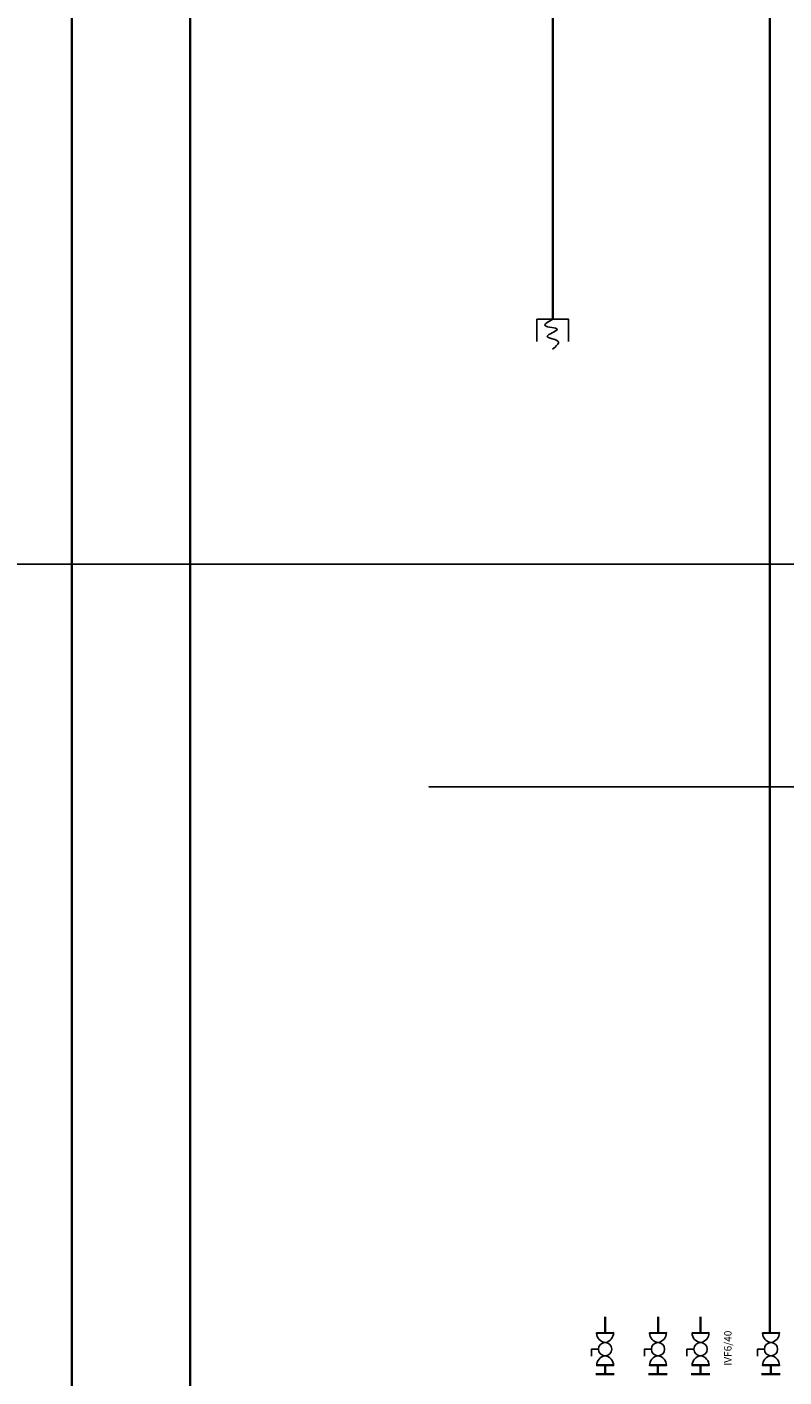
# Model space of a CAD drawing. Units: millimetres. Extents: x 353872 to 441597, y 126154 to 187356.
# Tile 11 of 28: x 381210 to 391248, y 149281 to 167178. Entities that reach past the tile are written whole.
import ezdxf

# ---------------------------------------------------------------- set-up
doc = ezdxf.new("R2010")
doc.units = ezdxf.units.MM
doc.linetypes.add('ACAD_ISO02W100', pattern=[15, 12, -3])
for name, color, linetype, lineweight in [('A-ANNO-DIMS', 2, 'Continuous', 18), ('P-ANNO-TEXT', 7, 'Continuous', 25), ('P-BNDY', 4, 'ACAD_ISO02W100', 25), ('P-PIPE', 3, 'Continuous', 35), ('P-VALV', 2, 'Continuous', 25)]:
    doc.layers.add(name, color=color, linetype=linetype, lineweight=lineweight)
doc.styles.get("Standard").update_dxf_attribs({"font": 'arial.ttf'})
doc.dimstyles.get("Standard").update_dxf_attribs({"dimtxt": 0.18, "dimasz": 0.18, "dimexe": 0.18, "dimexo": 0.0625, "dimgap": 0.09, "dimtad": 0, "dimtih": 1, "dimtoh": 1, "dimdec": 4, "dimzin": 0, "dimdsep": 46, "dimtxsty": 'Standard', "dimcen": 0.09, "dimadec": 0, "dimazin": 0, "dimtfac": 1, "dimtdec": 4, "dimtofl": 0, "dimtmove": 0, "dimatfit": 3, "dimfxl": 1, "dimtolj": 1, "dimtzin": 0, "dimarcsym": 0})

# ---------------------------------------------------------------- blocks, each defined once
blk = doc.blocks.new('VALVE-C')
for points in [[(0, 8), (224, 8)], [(0, 5), (224, 5)], [(0, 3), (0, 0), (224, 0), (224, 3)], [(0, 3), (0, 3), (222, 3), (224, 3)]]:
    blk.add_lwpolyline(points)
for centre, start, end in [((128, 1), 97.3612, 180.5798), ((96, 2), 359.2193, 82.8397)]:
    blk.add_arc(centre, 128, start, end)
blk = doc.blocks.new('*D34')
at = {"layer": 'A-ANNO-DIMS', "color": 0, "lineweight": -2, "transparency": 16777216}
for p, q in [((399457, 167930), (356736, 167930)), ((356737, 167930), (356737, 163994)), ((356737, 160058), (356737, 163994)), ((399457, 160058), (356736, 160058))]:
    blk.add_line(p, q, dxfattribs=at)
at = {"layer": 'A-ANNO-DIMS', "color": 0, "transparency": 16777216}
for points in [[(356737, 167930), (356737, 167930), (356737, 167930)], [(356737, 160058), (356737, 160058), (356737, 160058)]]:
    blk.add_solid(points, dxfattribs=at)
at = {"layer": 'Defpoints', "color": 0, "transparency": 16777216}
for p in [(399457, 167930), (356737, 160058), (399457, 160058)]:
    blk.add_point(p, dxfattribs=at)
at = {"layer": 'A-ANNO-DIMS', "color": 0, "transparency": 16777216, "insert": (356737, 163994), "char_height": 0.18, "attachment_point": 5}
blk.add_mtext('\\A1;7872', dxfattribs=at)

msp = doc.modelspace()

# ---------------------------------------------------------------- linework, layer by layer
at = {"layer": 'P-BNDY'}
msp.add_line((436591, 157104.68), (386532.91, 157104.68), dxfattribs=at)
at = {"layer": 'P-PIPE'}
for p, q in [((388876.24, 150079.91), (388876.24, 149867.25)), ((389577.76, 150079.91), (389577.76, 149867.25)), ((390142.2, 150079.91), (390142.2, 149867.25)), ((391060.3, 150079.91), (391060.3, 149867.25)), ((388996.7, 149319.73), (388751.94, 149319.73)), ((388874.98, 149433.14), (388874.98, 149319.73)), ((389698.22, 149319.73), (389453.46, 149319.73)), ((389576.5, 149433.14), (389576.5, 149319.73)), ((390262.67, 149319.73), (390017.91, 149319.73)), ((390140.95, 149433.14), (390140.95, 149319.73)), ((391196.72, 149319.73), (390951.96, 149319.73)), ((391075, 149433.14), (391075, 149319.73))]:
    msp.add_line(p, q, dxfattribs=at)
for points in [[(391060.3, 150079.91), (391060.3, 182028.44), (390103.2, 182028.44), (366976.76, 182028.44)], [(366976.76, 173434.34), (386613.67, 173434.34), (388181.19, 173434.34), (388181.19, 163303.71)], [(366976.76, 171744.89), (381803.29, 171744.89), (381803.29, 150820.94), (381803.29, 147742.48), (377889.79, 147742.48)]]:
    msp.add_lwpolyline(points, dxfattribs=at)
msp.add_lwpolyline([(388213.21, 147045.52), (383375.2, 147045.17), (383375.2, 147045.17), (383375.2, 149602.24), (383375.2, 167832.6), (382147.59, 167832.6, 1), (381458.98, 167832.6), (380124.81, 167832.6, 1), (379436.2, 167832.6), (368453.37, 167832.6)], format="xyb", dxfattribs=at)
at = {"layer": 'P-VALV'}
for points in [[(388391.21, 163010.43), (388391.21, 163303.71), (387971.17, 163303.71), (387971.17, 163010.43)], [(388787.65, 149650.19), (388695.2, 149650.19), (388695.2, 149559.43)], [(389489.17, 149650.19), (389396.73, 149650.19), (389396.73, 149559.43)], [(390053.62, 149650.19), (389961.17, 149650.19), (389961.17, 149559.43)], [(390987.67, 149650.19), (390895.22, 149650.19), (390895.22, 149559.43)]]:
    msp.add_lwpolyline(points, dxfattribs=at)
for centre in [(388875.94, 149650.19), (389577.46, 149650.19), (390141.91, 149650.19), (391075.95, 149650.19)]:
    msp.add_circle(centre, 88.29, dxfattribs=at)
msp.add_open_spline([(388181.19, 163303.71), (388122.73, 163271.25), (387989.49, 163197.29), (388375.07, 163190.34), (387981.2, 163061.46), (388331.17, 163032.41), (388225.96, 162945.08), (388179.78, 162906.75)], degree=3, knots=[0, 0, 0, 0, 131.62046813, 299.94883433, 460.08690619, 621.6605897, 748.04024912, 748.04024912, 748.04024912, 748.04024912], dxfattribs=at)

# ---------------------------------------------------------------- block references
for p, rotation in [((388987.77, 149869.79), 181.3019170023728), ((389689.29, 149869.79), 181.3019170023652), ((390253.73, 149869.79), 181.3019170023652), ((391187.78, 149869.79), 181.3019170023694)]:
    msp.add_blockref('VALVE-C', p, dxfattribs=dict(at, rotation=rotation))
for p in [(388764.22, 149433.14), (389465.74, 149433.14), (390030.19, 149433.14), (390964.24, 149433.14)]:
    msp.add_blockref('VALVE-C', p, dxfattribs=at)

# ---------------------------------------------------------------- texts
at = {"layer": 'P-ANNO-TEXT'}
msp.add_text('IVF6/40', height=98.09, rotation=90, dxfattribs=at).set_placement((390552.8, 149431.04))

# ---------------------------------------------------------------- dimensions: what is measured, and where the dimension line sits
at = {"layer": 'A-ANNO-DIMS'}
dim = msp.add_linear_dim(base=(356736.55, 160058.19), p1=(399457.15, 167929.97), p2=(399457.15, 160058.19), angle=90, dimstyle='Standard', override={"dimdec": 0, "dimlfac": 1, "dimrnd": 0, "dimzin": 0, "dimdsep": 46, "dimlunit": 2}, dxfattribs=at)
dim.commit()
dim.dimension.update_dxf_attribs({"geometry": '*D34', "text_midpoint": (356736.55, 163994.08)})

doc.saveas('drawing.dxf')
